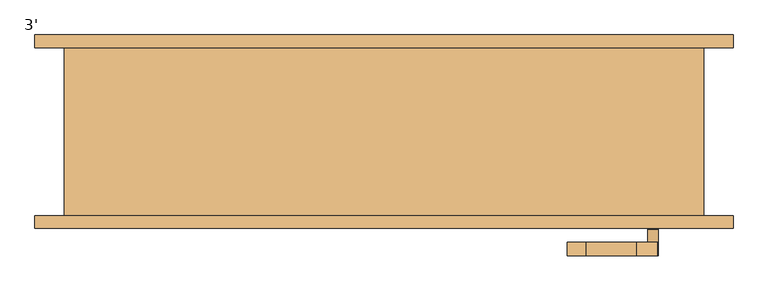
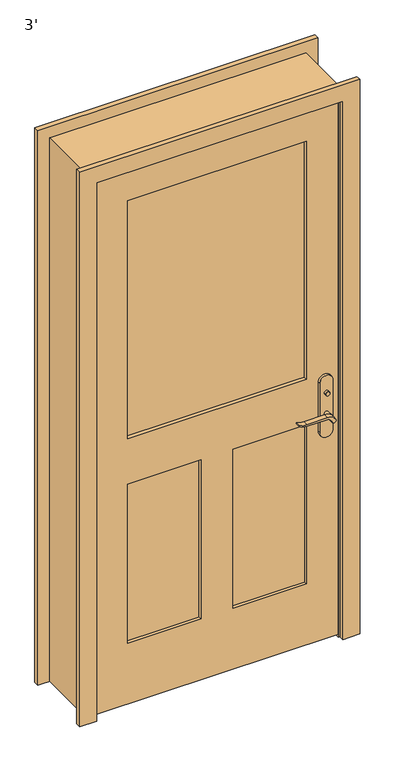
"""IFC4 building model written with IfcOpenShell, lengths in millimetres: door geometry, 3'."""

from ifc_helpers import new_model, si_unit, point, frame, frame_2d, origin, place, context, project, spatial, polyline, circle_curve, trimmed, segment, composite_curve, outline, extrude, faceted_brep, source, transform, mapped, element, save


def door_3_192038f1(model_context):
    return source(origin(), model_context, "Body", "SolidModel", [
        extrude(outline(polyline([(-38.1, 12.7), (-12.7, 0.0), (-98.425, 0.0), (-73.025, 12.7), (-38.1, 12.7)])), frame((-457.2, 0.0, 0.0), z_axis=(1.0, 0.0, 0.0), x_axis=(0.0, 1.0, 0.0)), (0.0, 0.0, 1.0), 914.4),
        extrude(outline(polyline([(411.4, -68.9), (411.4, -78.9), (401.4, -78.9), (401.4, -68.9), (411.4, -68.9)])), frame((0.0, 0.0, 981.9), z_axis=(0.0, 0.0, 1.0), x_axis=(1.0, 0.0, 0.0)), (0.0, 0.0, 1.0), 30.0),
        extrude(outline(composite_curve([segment(trimmed(circle_curve(frame_2d((996.9, 406.4)), 8.0), [point((996.9, 398.4))], [point((996.9, 414.4))], False, "CARTESIAN"), True, "CONTINUOUS"), segment(trimmed(circle_curve(frame_2d((996.9, 406.4)), 8.0), [point((996.9, 414.4))], [point((996.9, 398.4))], False, "CARTESIAN"), True, "CONTINUOUS")], self_intersect=False)), frame((0.0, -143.825, 0.0), z_axis=(0.0, 1.0, 0.0), x_axis=(0.0, 0.0, 1.0)), (0.0, 0.0, 1.0), 10.0),
        extrude(outline(composite_curve([segment(trimmed(circle_curve(frame_2d((897.1555521, 382.7324871)), 37.2832219), [point((919.0523287, 412.9081363))], [point((934.4, 381.0325667))], False, "CARTESIAN"), True, "CONTINUOUS"), segment(polyline([(934.4, 381.0325667), (934.4, 304.7564091)]), True, "CONTINUOUS"), segment(trimmed(circle_curve(frame_2d((1017.6850638, 304.8227909)), 83.2850902), [point((934.4, 304.7564091))], [point((939.4, 276.4))], True, "CARTESIAN"), True, "CONTINUOUS"), segment(polyline([(939.4, 276.4), (936.6135558, 276.4)]), True, "CONTINUOUS"), segment(trimmed(circle_curve(frame_2d((986.6709207, 308.3396612)), 59.3791355), [point((936.6135558, 276.4))], [point((927.4, 304.7564091))], False, "CARTESIAN"), True, "CONTINUOUS"), segment(polyline([(927.4, 304.7564091), (927.4, 381.0138099)]), True, "CONTINUOUS"), segment(trimmed(circle_curve(frame_2d((909.2738613, 381.0138099)), 18.1261387), [point((927.4, 381.0138099))], [point((914.4, 398.4))], True, "CARTESIAN"), True, "CONTINUOUS"), segment(trimmed(circle_curve(frame_2d((914.4, 406.4)), 8.0), [point((914.4, 398.4))], [point((919.0523287, 412.9081363))], False, "CARTESIAN"), True, "CONTINUOUS")], self_intersect=False)), frame((0.0, -48.9, 0.0), z_axis=(0.0, 1.0, 0.0), x_axis=(0.0, 0.0, 1.0)), (0.0, 0.0, 1.0), 20.0),
        extrude(outline(composite_curve([segment(trimmed(circle_curve(frame_2d((914.4, 406.4)), 8.0), [point((914.3999903, 398.4))], [point((919.0523287, 412.9081363))], False, "CARTESIAN"), True, "CONTINUOUS"), segment(trimmed(circle_curve(frame_2d((897.1555521, 382.7324871)), 37.2832219), [point((919.0523287, 412.9081363))], [point((934.4, 381.0325667))], False, "CARTESIAN"), True, "CONTINUOUS"), segment(polyline([(934.4, 381.0325667), (934.4, 304.7564091)]), True, "CONTINUOUS"), segment(trimmed(circle_curve(frame_2d((1017.6850638, 304.8227909)), 83.2850902), [point((934.4, 304.7564091))], [point((939.4, 276.4))], True, "CARTESIAN"), True, "CONTINUOUS"), segment(polyline([(939.4, 276.4), (936.6135558, 276.4)]), True, "CONTINUOUS"), segment(trimmed(circle_curve(frame_2d((986.6709207, 308.3396612)), 59.3791355), [point((936.6135558, 276.4))], [point((927.4, 304.7564091))], False, "CARTESIAN"), True, "CONTINUOUS"), segment(polyline([(927.4, 304.7564091), (927.4, 381.0138122)]), True, "CONTINUOUS"), segment(trimmed(circle_curve(frame_2d((909.2738682, 381.0138122)), 18.1261318), [point((927.4, 381.0138122))], [point((914.3999903, 398.4))], True, "CARTESIAN"), True, "CONTINUOUS")], self_intersect=False)), frame((0.0, -183.825, 0.0), z_axis=(0.0, 1.0, 0.0), x_axis=(0.0, 0.0, 1.0)), (0.0, 0.0, 1.0), 20.0),
        extrude(outline(composite_curve([segment(trimmed(circle_curve(frame_2d((914.4, 406.4)), 8.0), [point((914.4, 398.4))], [point((914.4, 414.4))], False, "CARTESIAN"), True, "CONTINUOUS"), segment(trimmed(circle_curve(frame_2d((914.4, 406.4)), 8.0), [point((914.4, 414.4))], [point((914.4, 398.4))], False, "CARTESIAN"), True, "CONTINUOUS")], self_intersect=False)), frame((0.0, -78.9, 0.0), z_axis=(0.0, 1.0, 0.0), x_axis=(0.0, 0.0, 1.0)), (0.0, 0.0, 1.0), 30.0),
        extrude(outline(composite_curve([segment(trimmed(circle_curve(frame_2d((914.4, 406.4)), 8.0), [point((914.4, 398.4))], [point((914.4, 414.4))], False, "CARTESIAN"), True, "CONTINUOUS"), segment(trimmed(circle_curve(frame_2d((914.4, 406.4)), 8.0), [point((914.4, 414.4))], [point((914.4, 398.4))], False, "CARTESIAN"), True, "CONTINUOUS")], self_intersect=False)), frame((0.0, -163.825, 0.0), z_axis=(0.0, 1.0, 0.0), x_axis=(0.0, 0.0, 1.0)), (0.0, 0.0, 1.0), 30.0),
        extrude(outline(composite_curve([segment(polyline([(844.4, 431.4), (1039.4, 431.4)]), True, "CONTINUOUS"), segment(trimmed(circle_curve(frame_2d((1039.4, 406.4)), 25.0), [point((1039.4, 431.4))], [point((1039.4, 381.4))], False, "CARTESIAN"), True, "CONTINUOUS"), segment(polyline([(1039.4, 381.4), (844.4, 381.4)]), True, "CONTINUOUS"), segment(trimmed(circle_curve(frame_2d((844.4, 406.4)), 25.0), [point((844.4, 381.4))], [point((844.4, 431.4))], False, "CARTESIAN"), True, "CONTINUOUS")], self_intersect=False)), frame((0.0, -88.9, 0.0), z_axis=(0.0, 1.0, 0.0), x_axis=(0.0, 0.0, 1.0)), (0.0, 0.0, 1.0), 10.0),
        extrude(outline(composite_curve([segment(polyline([(844.4, 431.4), (1039.4, 431.4)]), True, "CONTINUOUS"), segment(trimmed(circle_curve(frame_2d((1039.4, 406.4)), 25.0), [point((1039.4, 431.4))], [point((1039.4, 381.4))], False, "CARTESIAN"), True, "CONTINUOUS"), segment(polyline([(1039.4, 381.4), (844.4, 381.4)]), True, "CONTINUOUS"), segment(trimmed(circle_curve(frame_2d((844.4, 406.4)), 25.0), [point((844.4, 381.4))], [point((844.4, 431.4))], False, "CARTESIAN"), True, "CONTINUOUS")], self_intersect=False)), frame((0.0, -133.825, 0.0), z_axis=(0.0, 1.0, 0.0), x_axis=(0.0, 0.0, 1.0)), (0.0, 0.0, 1.0), 10.0),
        faceted_brep([(482.6, -123.825, 0.0), (457.2, -123.825, 0.0), (457.2, -88.9, 0.0), (444.5, -88.9, 0.0), (444.5, -53.975, 0.0), (457.2, -53.975, 0.0), (457.2, 130.175, 0.0), (482.6, 130.175, 0.0), (482.6, 130.175, 2159.0), (482.6, -123.825, 2159.0), (457.2, 130.175, 2133.6), (-457.2, 130.175, 2133.6), (-457.2, 130.175, 0.0), (-482.6, 130.175, 0.0), (-482.6, 130.175, 2159.0), (457.2, -53.975, 2133.6), (444.5, -53.975, 2120.9), (-444.5, -53.975, 2120.9), (-444.5, -53.975, 0.0), (-457.2, -53.975, 0.0), (-457.2, -53.975, 2133.6), (444.5, -88.9, 2120.9), (457.2, -88.9, 2133.6), (-457.2, -88.9, 2133.6), (-457.2, -88.9, 0.0), (-444.5, -88.9, 0.0), (-444.5, -88.9, 2120.9), (457.2, -123.825, 2133.6), (-482.6, -123.825, 2159.0), (-482.6, -123.825, 0.0), (-457.2, -123.825, 0.0), (-457.2, -123.825, 2133.6)], [[[0, 1, 2, 3, 4, 5, 6, 7]], [[7, 8, 9, 0]], [[6, 10, 11, 12, 13, 14, 8, 7]], [[5, 15, 10, 6]], [[4, 16, 17, 18, 19, 20, 15, 5]], [[3, 21, 16, 4]], [[2, 22, 23, 24, 25, 26, 21, 3]], [[1, 27, 22, 2]], [[0, 9, 28, 29, 30, 31, 27, 1]], [[8, 14, 28, 9]], [[15, 20, 11, 10]], [[21, 26, 17, 16]], [[27, 31, 23, 22]], [[29, 13, 12, 19, 18, 25, 24, 30]], [[14, 13, 29, 28]], [[20, 19, 12, 11]], [[26, 25, 18, 17]], [[31, 30, 24, 23]]]),
        extrude(outline(polyline([(2133.6, -457.2), (12.7, -457.2), (12.7, 457.2), (2133.6, 457.2), (2133.6, -457.2)]), holes=[polyline([(1066.8, -336.55), (2012.95, -336.55), (2012.95, 336.55), (1066.8, 336.55), (1066.8, -336.55)]), polyline([(885.825, -60.325), (254.0, -60.325), (254.0, -336.55), (885.825, -336.55), (885.825, -60.325)]), polyline([(885.825, 336.55), (254.0, 336.55), (254.0, 60.325), (885.825, 60.325), (885.825, 336.55)])]), frame((0.0, -123.825, 0.0), z_axis=(0.0, 1.0, 0.0), x_axis=(0.0, 0.0, 1.0)), (0.0, 0.0, 1.0), 34.925),
        extrude(outline(polyline([(336.55, -102.87), (336.55, -109.855), (-336.55, -109.855), (-336.55, -102.87), (336.55, -102.87)])), frame((0.0, 0.0, 1066.8), z_axis=(0.0, 0.0, 1.0), x_axis=(1.0, 0.0, 0.0)), (0.0, 0.0, 1.0), 946.15),
        extrude(outline(polyline([(-60.325, -100.5416667), (-60.325, -112.1833333), (-336.55, -112.1833333), (-336.55, -100.5416667), (-60.325, -100.5416667)])), frame((0.0, 0.0, 254.0), z_axis=(0.0, 0.0, 1.0), x_axis=(1.0, 0.0, 0.0)), (0.0, 0.0, 1.0), 631.825),
        extrude(outline(polyline([(336.55, -100.5416667), (336.55, -112.1833333), (60.325, -112.1833333), (60.325, -100.5416667), (336.55, -100.5416667)])), frame((0.0, 0.0, 254.0), z_axis=(0.0, 0.0, 1.0), x_axis=(1.0, 0.0, 0.0)), (0.0, 0.0, 1.0), 631.825),
        extrude(outline(polyline([(0.0, -463.55), (2139.95, -463.55), (2139.95, 463.55), (0.0, 463.55), (0.0, 527.05), (2203.45, 527.05), (2203.45, -527.05), (0.0, -527.05), (0.0, -463.55)])), frame((0.0, -142.875, 0.0), z_axis=(0.0, 1.0, 0.0), x_axis=(0.0, 0.0, 1.0)), (0.0, 0.0, 1.0), 19.05),
        extrude(outline(polyline([(0.0, -463.55), (2139.95, -463.55), (2139.95, 463.55), (0.0, 463.55), (0.0, 527.05), (2203.45, 527.05), (2203.45, -527.05), (0.0, -527.05), (0.0, -463.55)])), frame((0.0, 130.175, 0.0), z_axis=(0.0, 1.0, 0.0), x_axis=(0.0, 0.0, 1.0)), (0.0, 0.0, 1.0), 19.05),
    ])


if __name__ == "__main__":
    model = new_model("IFC4")
    model_context = context("Model", 3, world=origin())
    ifc_project = project(units=[si_unit("LENGTHUNIT", "METRE", prefix="MILLI")], contexts=[model_context])
    site = spatial("IfcSite", under=ifc_project)
    building = spatial("IfcBuilding", under=site)
    placement = place(None, origin())
    door_3_shape = door_3_192038f1(model_context)
    element("IfcDoor", 1, ObjectType="3'", at=placement, inside=building, context=model_context, shape_type="MappedRepresentation", body=[
        mapped(door_3_shape, transform((0.0, 0.0, 0.0), x_axis=(1.0, 0.0, 0.0), y_axis=(0.0, 1.0, 0.0), z_axis=(0.0, 0.0, 1.0))),
    ])
    save(model, "model.ifc")

# Revit data of these elements
# Type "3'"
#   Type Mark = "12"
#   Assembly Code = "B2030100"
#   Analytic Construction = "French door, wood frame with single glass"
#   Top Rail = 0' - 4 3/4"
#   Threshold Offset [instance default] = 0' - 0 1/2"
#   Thickness = 0' - 1 3/8"
#   Thermal Resistance (R) = 1.0696 (h·ft²·°F)/BTU
#   Swing Angle [instance default] = 90.00°
#   Stiles = 0' - 4 3/4"
#   Rough Width = 3' - 2"
#   Rough Height = 7' - 1"
#   Lock Rail = 0' - 7 1/8"
#   Height = 7' - 0"
#   Width = 3' - 0"
#   Heat Transfer Coefficient (U) = 0.9350 BTU/(h·ft²·°F)
#   Door Offset [instance default] = 0' - 0"
#   Bottom Rail = 0' - 9 1/2"
#   Threshold [instance default] = yes
#   Function = 1
#   Exterior Trim [instance default] = yes
#   Trim Material = Cherry
#   Threshold Material = Cherry
#   Panel Material = Cherry
#   Glazing = Glass
#   Frame Material = Cherry
#   Door Handle Material = Aluminum
#   Visual Light Transmittance = 0
#   Solar Heat Gain Coefficient = 0
#   Wall Closure = (empty or 0)
#   Construction Type = (empty or 0)
# Element 1 (IfcDoor, "3'")
#   Materials on its faces: "Cherry", "Aluminum", "Glass"
# Materials
#   "Cherry": class "Wood", colour RGB 226 177 128, transparency 0, Description = "Prunus Serotina", Cost = 0
#   "Glass": class "Glass", colour RGB 0 128 192, transparency 0.75, Description = "Soda Lime Glass", Cost = 0
#   "Aluminum": class "Metal", colour RGB 247 247 247, transparency 0, Description = "Aluminum 6061", Cost = 0
